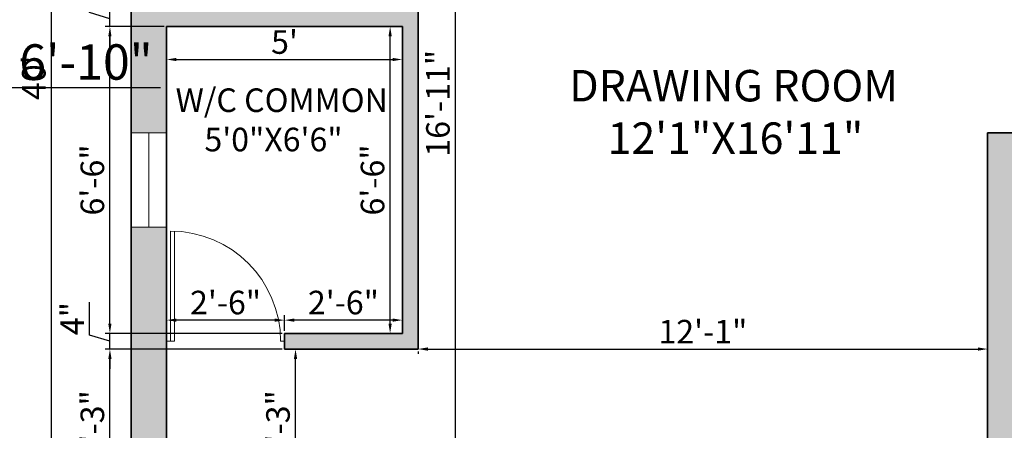
# Model space of a CAD drawing. Units: inches. Extents: x 3592 to 4861, y 1650 to 2243.
# Tile 27 of 30: x 4438 to 4688, y 1836 to 1940. Entities that reach past the tile are written whole.
import ezdxf

# ---------------------------------------------------------------- set-up
doc = ezdxf.new("R2010")
doc.units = ezdxf.units.IN
for name, color, linetype, lineweight in [('A-ANNO-DIMS', 2, 'Continuous', 13), ('A-AREA-IDEN', 7, 'Continuous', 18), ('A-DOOR', 3, 'Continuous', 20), ('A-GLAZ', 4, 'Continuous', 18), ('A-WALL', 7, 'Continuous', 35)]:
    doc.layers.add(name, color=color, linetype=linetype, lineweight=lineweight)
doc.layers.add('A-WALL-PATT', color=252, linetype='Continuous', lineweight=13, true_color=0x939598)
doc.styles.get("Standard").update_dxf_attribs({"font": 'arial.ttf'})
doc.dimstyles.new('ISO-25', dxfattribs={"dimtxt": 9, "dimasz": 2.5, "dimexe": 1.25, "dimexo": 0.625, "dimtad": 1, "dimlunit": 3, "dimtxsty": 'Standard', "dimcen": 2.5, "dimadec": 0, "dimazin": 0, "dimtfac": 1, "dimtmove": 0, "dimatfit": 3, "dimfxl": 1, "dimarcsym": 0})

# ---------------------------------------------------------------- blocks, each defined once
blk = doc.blocks.new('2')
for p, q in [((3637.19, 1914.49), (3637.19, 1942.49)), ((3638.19, 1914.49), (3638.19, 1942.49)), ((3636.19, 1914.49), (3638.19, 1914.49)), ((3665.19, 1914.49), (3666.19, 1914.49))]:
    blk.add_line(p, q)
blk.add_arc((3637.19, 1914.49), 28, 0, 90)
blk = doc.blocks.new('*D85')
at = {"layer": 'A-ANNO-DIMS', "color": 0, "lineweight": -2, "transparency": 16777216}
for p, q in [((4505.87, 1856.22), (4509.31, 1856.22)), ((4508.06, 1819.72), (4508.06, 1853.72)), ((4505.87, 1817.22), (4509.31, 1817.22))]:
    blk.add_line(p, q, dxfattribs=at)
at = {"layer": 'A-ANNO-DIMS', "color": 0, "transparency": 16777216}
for points in [[(4507.64, 1853.72), (4508.47, 1853.72), (4508.06, 1856.22)], [(4507.64, 1819.72), (4508.47, 1819.72), (4508.06, 1817.22)]]:
    blk.add_solid(points, dxfattribs=at)
at = {"layer": 'Defpoints', "color": 0, "transparency": 16777216}
for p in [(4505.25, 1856.22), (4508.06, 1856.22), (4505.25, 1817.22)]:
    blk.add_point(p, dxfattribs=at)
at = {"layer": 'A-ANNO-DIMS', "color": 0, "transparency": 16777216, "insert": (4504.37, 1836.72), "char_height": 6, "attachment_point": 5, "rotation": 90}
blk.add_mtext('3\'-3"', dxfattribs=at)
blk = doc.blocks.new('*D86')
at = {"layer": 'A-ANNO-DIMS', "color": 0, "lineweight": -2, "transparency": 16777216}
for p, q in [((4534.62, 1938.22), (4530.89, 1938.22)), ((4532.14, 1862.72), (4532.14, 1935.72)), ((4534.62, 1860.22), (4530.89, 1860.22))]:
    blk.add_line(p, q, dxfattribs=at)
at = {"layer": 'A-ANNO-DIMS', "color": 0, "transparency": 16777216}
for points in [[(4531.72, 1935.72), (4532.56, 1935.72), (4532.14, 1938.22)], [(4531.72, 1862.72), (4532.56, 1862.72), (4532.14, 1860.22)]]:
    blk.add_solid(points, dxfattribs=at)
at = {"layer": 'Defpoints', "color": 0, "transparency": 16777216}
for p in [(4532.14, 1938.22), (4535.25, 1938.22), (4535.25, 1860.22)]:
    blk.add_point(p, dxfattribs=at)
at = {"layer": 'A-ANNO-DIMS', "color": 0, "transparency": 16777216, "insert": (4528.45, 1899.22), "char_height": 6, "attachment_point": 5, "rotation": 90}
blk.add_mtext('6\'-6"', dxfattribs=at)
blk = doc.blocks.new('*D87')
at = {"layer": 'A-ANNO-DIMS', "color": 0, "lineweight": -2, "transparency": 16777216}
for p, q in [((4475.25, 1937.59), (4475.25, 1928.6)), ((4535.25, 1937.59), (4535.25, 1928.6)), ((4477.75, 1929.85), (4532.75, 1929.85))]:
    blk.add_line(p, q, dxfattribs=at)
at = {"layer": 'A-ANNO-DIMS', "color": 0, "transparency": 16777216}
for points in [[(4477.75, 1930.27), (4477.75, 1929.43), (4475.25, 1929.85)], [(4532.75, 1930.27), (4532.75, 1929.43), (4535.25, 1929.85)]]:
    blk.add_solid(points, dxfattribs=at)
at = {"layer": 'Defpoints', "color": 0, "transparency": 16777216}
for p in [(4475.25, 1938.22), (4535.25, 1938.22), (4535.25, 1929.85)]:
    blk.add_point(p, dxfattribs=at)
at = {"layer": 'A-ANNO-DIMS', "color": 0, "transparency": 16777216, "insert": (4505.25, 1933.52), "char_height": 6, "attachment_point": 5}
blk.add_mtext("5'", dxfattribs=at)
blk = doc.blocks.new('*D88')
at = {"layer": 'A-ANNO-DIMS', "color": 0, "lineweight": -2, "transparency": 16777216}
for p, q in [((4505.25, 1860.84), (4505.25, 1864.83)), ((4535.25, 1860.84), (4535.25, 1864.83)), ((4532.75, 1863.58), (4507.75, 1863.58))]:
    blk.add_line(p, q, dxfattribs=at)
at = {"layer": 'A-ANNO-DIMS', "color": 0, "transparency": 16777216}
for points in [[(4507.75, 1863.99), (4507.75, 1863.16), (4505.25, 1863.58)], [(4532.75, 1863.99), (4532.75, 1863.16), (4535.25, 1863.58)]]:
    blk.add_solid(points, dxfattribs=at)
at = {"layer": 'Defpoints', "color": 0, "transparency": 16777216}
for p in [(4505.25, 1863.58), (4505.25, 1860.22), (4535.25, 1860.22)]:
    blk.add_point(p, dxfattribs=at)
at = {"layer": 'A-ANNO-DIMS', "color": 0, "transparency": 16777216, "insert": (4520.25, 1867.27), "char_height": 6, "attachment_point": 5}
blk.add_mtext('2\'-6"', dxfattribs=at)
blk = doc.blocks.new('*D89')
at = {"layer": 'A-ANNO-DIMS', "color": 0, "lineweight": -2, "transparency": 16777216}
for p, q in [((4475.25, 1864.2), (4475.25, 1864.83)), ((4505.25, 1860.84), (4505.25, 1864.83)), ((4502.75, 1863.58), (4477.75, 1863.58))]:
    blk.add_line(p, q, dxfattribs=at)
at = {"layer": 'A-ANNO-DIMS', "color": 0, "transparency": 16777216}
for points in [[(4477.75, 1863.99), (4477.75, 1863.16), (4475.25, 1863.58)], [(4502.75, 1863.99), (4502.75, 1863.16), (4505.25, 1863.58)]]:
    blk.add_solid(points, dxfattribs=at)
at = {"layer": 'Defpoints', "color": 0, "transparency": 16777216}
for p in [(4475.25, 1863.58), (4475.25, 1863.58), (4505.25, 1860.22)]:
    blk.add_point(p, dxfattribs=at)
at = {"layer": 'A-ANNO-DIMS', "color": 0, "transparency": 16777216, "insert": (4490.25, 1867.27), "char_height": 6, "attachment_point": 5}
blk.add_mtext('2\'-6"', dxfattribs=at)
blk = doc.blocks.new('*D92')
at = {"layer": 'A-ANNO-DIMS', "color": 0, "lineweight": -2, "transparency": 16777216}
for p, q in [((4546.11, 2020.22), (4550.03, 2020.22)), ((4548.78, 1819.72), (4548.78, 2017.72)), ((4546.11, 1817.22), (4550.03, 1817.22))]:
    blk.add_line(p, q, dxfattribs=at)
at = {"layer": 'A-ANNO-DIMS', "color": 0, "transparency": 16777216}
for points in [[(4548.36, 2017.72), (4549.19, 2017.72), (4548.78, 2020.22)], [(4548.36, 1819.72), (4549.19, 1819.72), (4548.78, 1817.22)]]:
    blk.add_solid(points, dxfattribs=at)
at = {"layer": 'Defpoints', "color": 0, "transparency": 16777216}
for p in [(4545.48, 2020.22), (4548.78, 2020.22), (4545.48, 1817.22)]:
    blk.add_point(p, dxfattribs=at)
at = {"layer": 'A-ANNO-DIMS', "color": 0, "transparency": 16777216, "insert": (4545.09, 1918.72), "char_height": 6, "attachment_point": 5, "rotation": 90}
blk.add_mtext('16\'-11"', dxfattribs=at)
blk = doc.blocks.new('*D93')
at = {"layer": 'A-ANNO-DIMS', "color": 0, "lineweight": -2, "transparency": 16777216}
for p, q in [((4684.25, 1856.84), (4684.25, 1857.47)), ((4539.25, 1855.59), (4539.25, 1854.97)), ((4541.75, 1856.22), (4681.75, 1856.22))]:
    blk.add_line(p, q, dxfattribs=at)
at = {"layer": 'A-ANNO-DIMS', "color": 0, "transparency": 16777216}
for points in [[(4541.75, 1856.64), (4541.75, 1855.8), (4539.25, 1856.22)], [(4681.75, 1856.64), (4681.75, 1855.8), (4684.25, 1856.22)]]:
    blk.add_solid(points, dxfattribs=at)
at = {"layer": 'Defpoints', "color": 0, "transparency": 16777216}
for p in [(4539.25, 1856.22), (4684.25, 1856.22), (4684.25, 1856.22)]:
    blk.add_point(p, dxfattribs=at)
at = {"layer": 'A-ANNO-DIMS', "color": 0, "transparency": 16777216, "insert": (4611.75, 1859.86), "char_height": 6, "attachment_point": 5}
blk.add_mtext('12\'-1"', dxfattribs=at)
blk = doc.blocks.new('*D103')
at = {"layer": 'A-ANNO-DIMS', "color": 0, "lineweight": -2, "transparency": 16777216}
for p, q in [((4504.62, 1856.22), (4459.56, 1856.22)), ((4460.81, 1819.72), (4460.81, 1853.72)), ((4504.62, 1817.22), (4459.56, 1817.22))]:
    blk.add_line(p, q, dxfattribs=at)
at = {"layer": 'A-ANNO-DIMS', "color": 0, "transparency": 16777216}
for points in [[(4460.39, 1853.72), (4461.22, 1853.72), (4460.81, 1856.22)], [(4460.39, 1819.72), (4461.22, 1819.72), (4460.81, 1817.22)]]:
    blk.add_solid(points, dxfattribs=at)
at = {"layer": 'Defpoints', "color": 0, "transparency": 16777216}
for p in [(4460.81, 1856.22), (4505.25, 1856.22), (4505.25, 1817.22)]:
    blk.add_point(p, dxfattribs=at)
at = {"layer": 'A-ANNO-DIMS', "color": 0, "transparency": 16777216, "insert": (4457.12, 1836.72), "char_height": 6, "attachment_point": 5, "rotation": 90}
blk.add_mtext('3\'-3"', dxfattribs=at)
blk = doc.blocks.new('*D104')
at = {"layer": 'A-ANNO-DIMS', "color": 0, "lineweight": -2, "transparency": 16777216}
for p, q in [((4455.62, 1859.78), (4455.62, 1868.16)), ((4460.81, 1862.72), (4460.81, 1865.22)), ((4504.62, 1860.22), (4459.56, 1860.22)), ((4460.81, 1856.22), (4460.81, 1860.22)), ((4460.81, 1856.22), (4460.81, 1860.22)), ((4460.81, 1858.22), (4455.62, 1859.78)), ((4504.62, 1856.22), (4459.56, 1856.22)), ((4460.81, 1853.72), (4460.81, 1851.22))]:
    blk.add_line(p, q, dxfattribs=at)
at = {"layer": 'A-ANNO-DIMS', "color": 0, "transparency": 16777216}
for points in [[(4460.39, 1862.72), (4461.22, 1862.72), (4460.81, 1860.22)], [(4460.39, 1853.72), (4461.22, 1853.72), (4460.81, 1856.22)]]:
    blk.add_solid(points, dxfattribs=at)
at = {"layer": 'Defpoints', "color": 0, "transparency": 16777216}
for p in [(4460.81, 1860.22), (4505.25, 1860.22), (4505.25, 1856.22)]:
    blk.add_point(p, dxfattribs=at)
at = {"layer": 'A-ANNO-DIMS', "color": 0, "transparency": 16777216, "insert": (4451.99, 1863.97), "char_height": 6, "attachment_point": 5, "rotation": 90}
blk.add_mtext('4"', dxfattribs=at)
blk = doc.blocks.new('*D105')
at = {"layer": 'A-ANNO-DIMS', "color": 0, "lineweight": -2, "transparency": 16777216}
for p, q in [((4474.62, 1938.22), (4459.56, 1938.22)), ((4460.81, 1862.72), (4460.81, 1935.72)), ((4504.62, 1860.22), (4459.56, 1860.22))]:
    blk.add_line(p, q, dxfattribs=at)
at = {"layer": 'A-ANNO-DIMS', "color": 0, "transparency": 16777216}
for points in [[(4460.39, 1935.72), (4461.22, 1935.72), (4460.81, 1938.22)], [(4460.39, 1862.72), (4461.22, 1862.72), (4460.81, 1860.22)]]:
    blk.add_solid(points, dxfattribs=at)
at = {"layer": 'Defpoints', "color": 0, "transparency": 16777216}
for p in [(4460.81, 1938.22), (4475.25, 1938.22), (4505.25, 1860.22)]:
    blk.add_point(p, dxfattribs=at)
at = {"layer": 'A-ANNO-DIMS', "color": 0, "transparency": 16777216, "insert": (4457.12, 1899.22), "char_height": 6, "attachment_point": 5, "rotation": 90}
blk.add_mtext('6\'-6"', dxfattribs=at)
blk = doc.blocks.new('*D106')
at = {"layer": 'A-ANNO-DIMS', "color": 0, "lineweight": -2, "transparency": 16777216}
for p, q in [((4455.62, 1941.78), (4455.62, 1950.16)), ((4460.81, 1944.72), (4460.81, 1947.22)), ((4460.81, 1940.22), (4455.62, 1941.78)), ((4474.62, 1942.22), (4459.56, 1942.22)), ((4460.81, 1938.22), (4460.81, 1942.22)), ((4460.81, 1938.22), (4460.81, 1942.22)), ((4474.62, 1938.22), (4459.56, 1938.22)), ((4460.81, 1935.72), (4460.81, 1933.22))]:
    blk.add_line(p, q, dxfattribs=at)
at = {"layer": 'A-ANNO-DIMS', "color": 0, "transparency": 16777216}
for points in [[(4460.39, 1944.72), (4461.22, 1944.72), (4460.81, 1942.22)], [(4460.39, 1935.72), (4461.22, 1935.72), (4460.81, 1938.22)]]:
    blk.add_solid(points, dxfattribs=at)
at = {"layer": 'Defpoints', "color": 0, "transparency": 16777216}
for p in [(4460.81, 1942.22), (4475.25, 1942.22), (4475.25, 1938.22)]:
    blk.add_point(p, dxfattribs=at)
at = {"layer": 'A-ANNO-DIMS', "color": 0, "transparency": 16777216, "insert": (4451.99, 1945.97), "char_height": 6, "attachment_point": 5, "rotation": 90}
blk.add_mtext('4"', dxfattribs=at)
blk = doc.blocks.new('*D131')
at = {"layer": 'A-ANNO-DIMS', "color": 0, "lineweight": -2, "transparency": 16777216}
for p, q in [((4465.62, 2165.22), (4444.65, 2165.22)), ((4445.9, 1687.72), (4445.9, 2162.72)), ((4465.62, 1685.22), (4444.65, 1685.22))]:
    blk.add_line(p, q, dxfattribs=at)
at = {"layer": 'A-ANNO-DIMS', "color": 0, "transparency": 16777216}
for points in [[(4445.49, 2162.72), (4446.32, 2162.72), (4445.9, 2165.22)], [(4445.49, 1687.72), (4446.32, 1687.72), (4445.9, 1685.22)]]:
    blk.add_solid(points, dxfattribs=at)
at = {"layer": 'Defpoints', "color": 0, "transparency": 16777216}
for p in [(4445.9, 2165.22), (4466.25, 2165.22), (4466.25, 1685.22)]:
    blk.add_point(p, dxfattribs=at)
at = {"layer": 'A-ANNO-DIMS', "color": 0, "transparency": 16777216, "insert": (4442.21, 1925.22), "char_height": 6, "attachment_point": 5, "rotation": 90}
blk.add_mtext("40'", dxfattribs=at)
blk = doc.blocks.new('*D158')
at = {"layer": 'A-ANNO-DIMS', "color": 0, "lineweight": -2, "transparency": 16777216}
for p, q in [((4281.9, 1934.46), (4281.9, 1921.52)), ((4364, 1934.46), (4364, 1921.52)), ((4284.4, 1922.77), (4361.5, 1922.77)), ((4364, 1922.77), (4473.66, 1922.77))]:
    blk.add_line(p, q, dxfattribs=at)
at = {"layer": 'A-ANNO-DIMS', "color": 0, "transparency": 16777216}
for points in [[(4284.4, 1923.19), (4284.4, 1922.36), (4281.9, 1922.77)], [(4361.5, 1923.19), (4361.5, 1922.36), (4364, 1922.77)]]:
    blk.add_solid(points, dxfattribs=at)
at = {"layer": 'Defpoints', "color": 0, "transparency": 16777216}
for p in [(4281.9, 1935.09), (4364, 1935.09), (4364, 1922.77)]:
    blk.add_point(p, dxfattribs=at)
at = {"layer": 'A-ANNO-DIMS', "color": 0, "transparency": 16777216, "insert": (4420.08, 1928.05), "char_height": 9, "attachment_point": 5}
blk.add_mtext('DINING SET 6\'-10"', dxfattribs=at)

msp = doc.modelspace()

# ---------------------------------------------------------------- hatches: boundary and pattern name
at = {"layer": 'A-WALL-PATT'}
h = msp.add_hatch(color=256, dxfattribs=at)
h.dxf.hatch_style = 1
h.paths.add_polyline_path([(4466.25, 2165.219), (4466.25, 1993.219), (4475.25, 1993.219), (4475.25, 2156.219), (4619.25, 2156.219), (4619.25, 2150.219), (4623.25, 2150.219), (4623.25, 2156.219), (4684.25, 2156.219), (4684.25, 2150.219), (4693.25, 2150.219), (4693.25, 2156.219), (4817.25, 2156.219), (4817.25, 2114.219), (4826.25, 2114.219), (4826.25, 2165.219)])
h.paths.add_polyline_path([(4623.25, 2096.219), (4623.25, 2102.219), (4619.25, 2102.219), (4619.25, 2020.219), (4623.25, 2020.219), (4623.25, 2087.219), (4684.25, 2087.219), (4684.25, 2020.219), (4734.25, 2020.219), (4734.25, 2024.219), (4693.25, 2024.219), (4693.25, 2102.219), (4684.25, 2102.219), (4684.25, 2096.219)], flags=17)
h.paths.add_polyline_path([(4817.25, 2024.219), (4776.25, 2024.219), (4776.25, 2020.219), (4817.25, 2020.219), (4817.25, 1989.719), (4826.25, 1989.719), (4826.25, 2066.219), (4817.25, 2066.219)])
h.paths.add_polyline_path([(4817.25, 1865.219), (4826.25, 1865.219), (4826.25, 1941.719), (4817.25, 1941.719), (4817.25, 1911.219), (4729.25, 1911.219), (4729.25, 1907.219), (4817.25, 1907.219)])
h.paths.add_polyline_path([(4826.25, 1817.219), (4817.25, 1817.219), (4817.25, 1775.219), (4693.25, 1775.219), (4693.25, 1911.219), (4684.25, 1911.219), (4684.25, 1817.219), (4648.75, 1817.219), (4648.75, 1808.219), (4684.25, 1808.219), (4684.25, 1766.219), (4817.25, 1766.219), (4817.25, 1694.219), (4684.25, 1694.219), (4684.25, 1685.219), (4826.25, 1685.219)])
h.paths.add_polyline_path([(4505.25, 1817.219), (4505.25, 1808.219), (4606.75, 1808.219), (4606.75, 1817.219)])
h.paths.add_polyline_path([(4539.25, 1856.219), (4539.25, 2020.219), (4583.25, 2020.219), (4583.25, 2024.219), (4505.25, 2024.219), (4505.25, 2020.219), (4535.25, 2020.219), (4535.25, 1942.219), (4475.25, 1942.219), (4475.25, 1969.219), (4466.25, 1969.219), (4466.25, 1911.219), (4475.25, 1911.219), (4475.25, 1938.219), (4535.25, 1938.219), (4535.25, 1860.219), (4505.25, 1860.219), (4505.25, 1856.219)])
h.paths.add_polyline_path([(4475.25, 1887.219), (4466.25, 1887.219), (4466.25, 1685.219), (4580.25, 1685.219), (4580.25, 1715.219), (4571.25, 1715.219), (4571.25, 1694.219), (4475.25, 1694.219)])
h.paths.add_polyline_path([(4571.25, 1751.219), (4580.25, 1751.219), (4580.25, 1772.219), (4571.25, 1772.219)], flags=17)

# ---------------------------------------------------------------- linework, layer by layer
at = {"layer": 'A-GLAZ'}
for p, q in [((4475.25, 1911.219), (4466.25, 1911.219)), ((4470.75, 1911.219), (4470.75, 1887.219)), ((4475.25, 1887.219), (4466.25, 1887.219))]:
    msp.add_line(p, q, dxfattribs=at)
at = {"layer": 'A-WALL'}
for p, q in [((4466.25, 1685.219), (4466.25, 2165.219)), ((4539.25, 1856.219), (4539.25, 2020.219)), ((4475.25, 1938.219), (4535.25, 1938.219)), ((4475.25, 1694.219), (4475.25, 1938.219)), ((4535.25, 1860.219), (4535.25, 1938.219)), ((4684.25, 1911.219), (4684.25, 1817.219)), ((4693.25, 1911.219), (4684.25, 1911.219)), ((4505.25, 1860.219), (4535.25, 1860.219)), ((4505.25, 1856.219), (4505.25, 1860.219)), ((4505.25, 1856.219), (4539.25, 1856.219))]:
    msp.add_line(p, q, dxfattribs=at)

# ---------------------------------------------------------------- block references
at = {"layer": 'A-DOOR'}
msp.add_blockref('2', (839.061, -56.273), dxfattribs=at)

# ---------------------------------------------------------------- texts
at = {"layer": 'A-AREA-IDEN', "attachment_point": 1}
for s, width, insert, char_height in [('DRAWING ROOM\\P    12\'1"X16\'11"', 142.74418, (4577.73, 1927.191), 8), ('W/C COMMON\\P    5\'0"X6\'6"', 121.44943, (4477.528, 1922.501), 6)]:
    msp.add_mtext_dynamic_manual_height_columns(s, width=width, gutter_width=12.5, heights=[0], dxfattribs=dict(at, insert=insert, char_height=char_height))

# ---------------------------------------------------------------- dimensions: what is measured, and where the dimension line sits
at = {"layer": 'A-ANNO-DIMS'}
for base, p1, p2, override, picture, middle in [((4445.902, 2165.219), (4466.25, 1685.219), (4466.25, 2165.219), {"dimtxt": 6, "dimclrd": 0, "dimclre": 0, "dimclrt": 0}, '*D131', (4442.214, 1925.219)), ((4548.776, 2020.219), (4545.484, 1817.219), (4545.484, 2020.219), {"dimtxt": 6, "dimclrd": 0, "dimclre": 0, "dimclrt": 0}, '*D92', (4545.088, 1918.719)), ((4460.807, 1942.219), (4475.25, 1938.219), (4475.25, 1942.219), {"dimtxt": 6, "dimclrd": 0, "dimclre": 0, "dimclrt": 0, "dimtmove": 1}, '*D106', (4451.994, 1942.4)), ((4460.807, 1938.219), (4505.25, 1860.219), (4475.25, 1938.219), {"dimtxt": 6, "dimclrd": 0, "dimclre": 0, "dimclrt": 0, "dimtmove": 1}, '*D105', (4457.118, 1899.219)), ((4532.139, 1938.219), (4535.25, 1860.219), (4535.25, 1938.219), {"dimtxt": 6, "dimclrd": 0, "dimclre": 0, "dimclrt": 0}, '*D86', (4528.45, 1899.219)), ((4460.807, 1860.219), (4505.25, 1856.219), (4505.25, 1860.219), {"dimtxt": 6, "dimclrd": 0, "dimclre": 0, "dimclrt": 0, "dimtmove": 1}, '*D104', (4451.994, 1860.4)), ((4460.807, 1856.219), (4505.25, 1817.219), (4505.25, 1856.219), {"dimtxt": 6, "dimclrd": 0, "dimclre": 0, "dimclrt": 0, "dimtmove": 1}, '*D103', (4457.116, 1836.719)), ((4508.058, 1856.219), (4505.25, 1817.219), (4505.25, 1856.219), {"dimtxt": 6, "dimclrd": 0, "dimclre": 0, "dimclrt": 0}, '*D85', (4504.368, 1836.719))]:
    dim = msp.add_linear_dim(base=base, p1=p1, p2=p2, angle=90, dimstyle='ISO-25', override=override, dxfattribs=at)
    dim.commit()
    dim.dimension.update_dxf_attribs({"geometry": picture, "text_midpoint": middle})
dim = msp.add_linear_dim(base=(4363.996, 1922.774), p1=(4281.898, 1935.089), p2=(4363.996, 1935.089), text='DINING SET <>', dimstyle='ISO-25', override={"dimdec": 1, "dimlfac": 1, "dimrnd": 0, "dimzin": 1, "dimdsep": 46, "dimlunit": 4, "dimfrac": 2}, dxfattribs=at)
dim.commit()
dim.dimension.update_dxf_attribs({"geometry": '*D158', "text_midpoint": (4420.077, 1928.052)})
for base, p1, p2, override, picture, middle in [((4535.25, 1929.848), (4475.25, 1938.219), (4535.25, 1938.219), {"dimtxt": 6, "dimclrd": 0, "dimclre": 0, "dimclrt": 0}, '*D87', (4505.25, 1933.525)), ((4475.25, 1863.577), (4505.25, 1860.219), (4475.25, 1863.577), {"dimtxt": 6, "dimclrd": 0, "dimclre": 0, "dimclrt": 0, "dimtmove": 1}, '*D89', (4490.25, 1867.266)), ((4505.25, 1863.577), (4535.25, 1860.219), (4505.25, 1860.219), {"dimtxt": 6, "dimclrd": 0, "dimclre": 0, "dimclrt": 0}, '*D88', (4520.25, 1867.266)), ((4684.25, 1856.219), (4539.25, 1856.219), (4684.25, 1856.219), {"dimtxt": 6, "dimclrd": 0, "dimclre": 0, "dimclrt": 0}, '*D93', (4611.75, 1859.856))]:
    dim = msp.add_linear_dim(base=base, p1=p1, p2=p2, dimstyle='ISO-25', override=override, dxfattribs=at)
    dim.commit()
    dim.dimension.update_dxf_attribs({"geometry": picture, "text_midpoint": middle})

doc.saveas('drawing.dxf')
